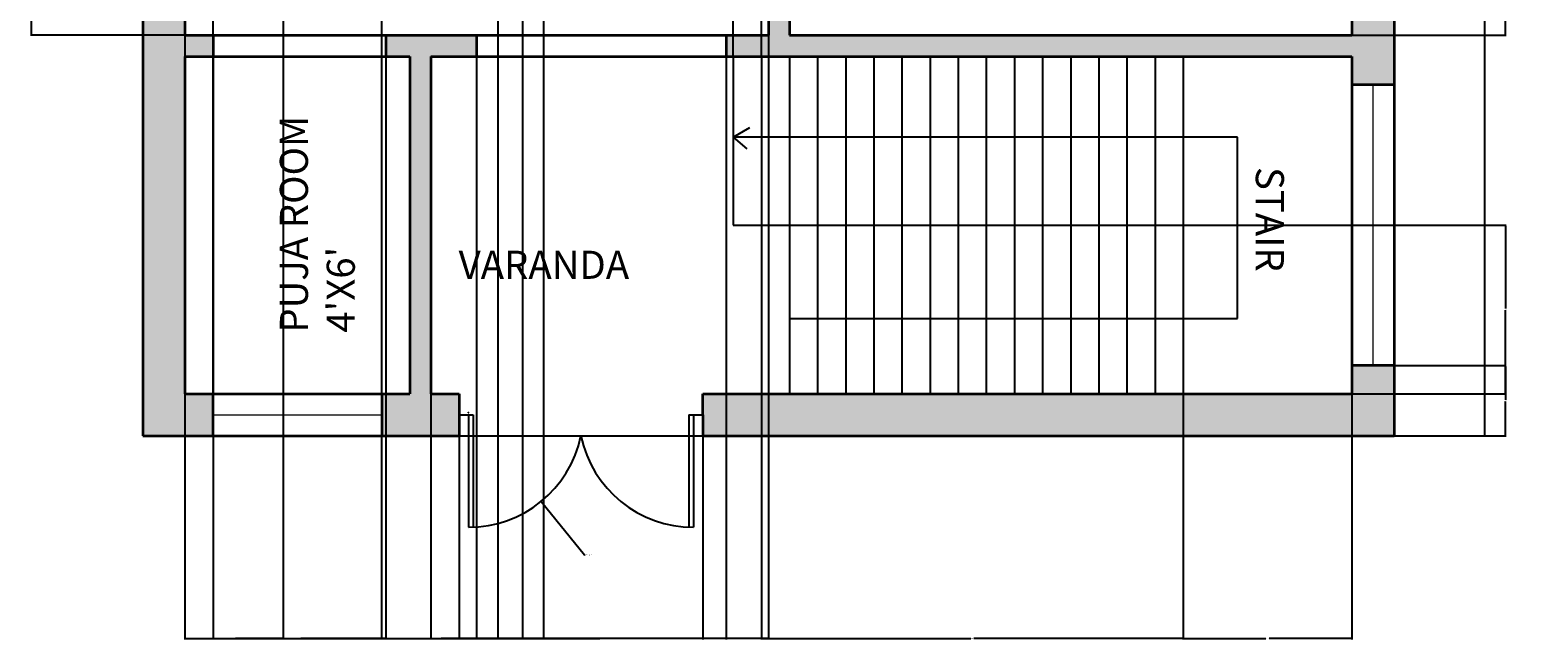
# Model space of a CAD drawing. Units: inches. Extents: x 10 to 332, y -471 to 73.
# Tile 1 of 5: x 10 to 332, y -471 to -341. Entities that reach past the tile are written whole.
import ezdxf

# ---------------------------------------------------------------- set-up
doc = ezdxf.new("R2010")
doc.units = ezdxf.units.IN
doc.header["$MEASUREMENT"] = 0
for name, color, linetype, lineweight in [('A-ANNO-DIMS', 2, 'Continuous', 18), ('A-AREA-IDEN', 7, 'Continuous', 18), ('A-DOOR', 3, 'Continuous', 25), ('A-FLOR-STRS', 7, 'Continuous', 25), ('A-GLAZ', 4, 'Continuous', 18), ('A-WALL', 7, 'Continuous', 35), ('A-WALL-PATT', 8, 'Continuous', 13)]:
    doc.layers.add(name, color=color, linetype=linetype, lineweight=lineweight)
doc.styles.get("Standard").update_dxf_attribs({"font": 'arial.ttf'})
doc.dimstyles.get("Standard").update_dxf_attribs({"dimtxt": 0.18, "dimasz": 0.18, "dimexe": 0.18, "dimexo": 0.0625, "dimgap": 0.09, "dimtad": 0, "dimtih": 1, "dimtoh": 1, "dimdec": 0, "dimzin": 0, "dimdsep": 46, "dimlunit": 3, "dimtxsty": 'Standard', "dimcen": 0.09, "dimadec": 0, "dimazin": 0, "dimtfac": 1, "dimtdec": 0, "dimtofl": 0, "dimtmove": 0, "dimatfit": 3, "dimfxl": 1, "dimtolj": 1, "dimtzin": 0, "dimarcsym": 0})

# ---------------------------------------------------------------- blocks, each defined once
blk = doc.blocks.new('*D3')
at = {"layer": 'A-ANNO-DIMS', "color": 0, "lineweight": -2, "transparency": 16777216}
for p, q in [((301.43, 11.99), (320.92, 11.99)), ((320.74, 11.81), (320.74, -204.61)), ((320.74, -427.33), (320.74, -210.92)), ((301.43, -427.51), (320.92, -427.51))]:
    blk.add_line(p, q, dxfattribs=at)
at = {"layer": 'A-ANNO-DIMS', "color": 0, "transparency": 16777216}
for points in [[(320.71, 11.81), (320.77, 11.81), (320.74, 11.99)], [(320.71, -427.33), (320.77, -427.33), (320.74, -427.51)]]:
    blk.add_solid(points, dxfattribs=at)
at = {"layer": 'Defpoints', "color": 0, "transparency": 16777216}
for p in [(301.37, 11.99), (301.37, -427.51), (320.74, -427.51)]:
    blk.add_point(p, dxfattribs=at)
at = {"layer": 'A-ANNO-DIMS', "color": 0, "transparency": 16777216, "insert": (320.74, -207.76), "char_height": 6, "attachment_point": 5}
blk.add_mtext('\\A1;36\'-8"', dxfattribs=at)
blk = doc.blocks.new('WIN-60')
for p, q in [((0, 9), (60, 9)), ((0, 4.5), (60, 4.5)), ((60, 0), (0, 0))]:
    blk.add_line(p, q)
blk = doc.blocks.new('*D30')
at = {"layer": 'A-ANNO-DIMS', "color": 0, "lineweight": -2, "transparency": 16777216}
for p, q in [((167.87, -93.08), (167.87, -470.94)), ((43.37, -97.58), (43.37, -470.94)), ((43.55, -470.76), (105.02, -470.76)), ((167.69, -470.76), (106.22, -470.76))]:
    blk.add_line(p, q, dxfattribs=at)
at = {"layer": 'A-ANNO-DIMS', "color": 0, "transparency": 16777216}
for points in [[(43.55, -470.73), (43.55, -470.79), (43.37, -470.76)], [(167.69, -470.73), (167.69, -470.79), (167.87, -470.76)]]:
    blk.add_solid(points, dxfattribs=at)
at = {"layer": 'Defpoints', "color": 0, "transparency": 16777216}
for p in [(167.87, -93.01), (43.37, -97.51), (167.87, -470.76)]:
    blk.add_point(p, dxfattribs=at)
at = {"layer": 'A-ANNO-DIMS', "color": 0, "transparency": 16777216, "insert": (105.62, -470.76), "char_height": 0.18, "attachment_point": 5}
blk.add_mtext('\\A1;10\'-4 1/2"', dxfattribs=at)
blk = doc.blocks.new('*D31')
at = {"layer": 'A-ANNO-DIMS', "color": 0, "lineweight": -2, "transparency": 16777216}
for p, q in [((43.3, -225.2), (10.44, -225.2)), ((10.62, -225.38), (10.62, -283.43)), ((10.62, -341.83), (10.62, -283.79)), ((43.3, -342.01), (10.44, -342.01))]:
    blk.add_line(p, q, dxfattribs=at)
at = {"layer": 'A-ANNO-DIMS', "color": 0, "transparency": 16777216}
for points in [[(10.59, -225.38), (10.65, -225.38), (10.62, -225.2)], [(10.59, -341.83), (10.65, -341.83), (10.62, -342.01)]]:
    blk.add_solid(points, dxfattribs=at)
at = {"layer": 'Defpoints', "color": 0, "transparency": 16777216}
for p in [(43.37, -225.2), (10.62, -342.01), (43.37, -342.01)]:
    blk.add_point(p, dxfattribs=at)
at = {"layer": 'A-ANNO-DIMS', "color": 0, "transparency": 16777216, "insert": (10.62, -283.61), "char_height": 0.18, "attachment_point": 5}
blk.add_mtext('\\A1;9\'-9"', dxfattribs=at)
blk = doc.blocks.new('*D32')
at = {"layer": 'A-ANNO-DIMS', "color": 0, "lineweight": -2, "transparency": 16777216}
for p, q in [((101.87, -427.58), (101.87, -470.94)), ((153.87, -427.58), (153.87, -470.94)), ((102.05, -470.76), (127.53, -470.76)), ((153.69, -470.76), (128.2, -470.76))]:
    blk.add_line(p, q, dxfattribs=at)
at = {"layer": 'A-ANNO-DIMS', "color": 0, "transparency": 16777216}
for points in [[(102.05, -470.73), (102.05, -470.79), (101.87, -470.76)], [(153.69, -470.73), (153.69, -470.79), (153.87, -470.76)]]:
    blk.add_solid(points, dxfattribs=at)
at = {"layer": 'Defpoints', "color": 0, "transparency": 16777216}
for p in [(101.87, -427.51), (153.87, -427.51), (153.87, -470.76)]:
    blk.add_point(p, dxfattribs=at)
at = {"layer": 'A-ANNO-DIMS', "color": 0, "transparency": 16777216, "insert": (127.87, -470.76), "char_height": 0.18, "attachment_point": 5}
blk.add_mtext('\\A1;4\'-4"', dxfattribs=at)
blk = doc.blocks.new('*D33')
at = {"layer": 'A-ANNO-DIMS', "color": 0, "lineweight": -2, "transparency": 16777216}
for p, q in [((95.87, -418.58), (95.87, -470.94)), ((101.87, -418.58), (101.87, -470.94)), ((96.05, -470.76), (98.54, -470.76)), ((101.69, -470.76), (99.2, -470.76))]:
    blk.add_line(p, q, dxfattribs=at)
at = {"layer": 'A-ANNO-DIMS', "color": 0, "transparency": 16777216}
for points in [[(96.05, -470.73), (96.05, -470.79), (95.87, -470.76)], [(101.69, -470.73), (101.69, -470.79), (101.87, -470.76)]]:
    blk.add_solid(points, dxfattribs=at)
at = {"layer": 'Defpoints', "color": 0, "transparency": 16777216}
for p in [(95.87, -418.51), (101.87, -418.51), (101.87, -470.76)]:
    blk.add_point(p, dxfattribs=at)
at = {"layer": 'A-ANNO-DIMS', "color": 0, "transparency": 16777216, "insert": (98.87, -470.76), "char_height": 0.18, "attachment_point": 5}
blk.add_mtext('\\A1;0\'-6"', dxfattribs=at)
blk = doc.blocks.new('*D34')
at = {"layer": 'A-ANNO-DIMS', "color": 0, "lineweight": -2, "transparency": 16777216}
for p, q in [((166.37, -418.58), (166.37, -470.94)), ((256.37, -418.58), (256.37, -470.94)), ((166.55, -470.76), (211.04, -470.76)), ((256.19, -470.76), (211.69, -470.76))]:
    blk.add_line(p, q, dxfattribs=at)
at = {"layer": 'A-ANNO-DIMS', "color": 0, "transparency": 16777216}
for points in [[(166.55, -470.73), (166.55, -470.79), (166.37, -470.76)], [(256.19, -470.73), (256.19, -470.79), (256.37, -470.76)]]:
    blk.add_solid(points, dxfattribs=at)
at = {"layer": 'Defpoints', "color": 0, "transparency": 16777216}
for p in [(166.37, -418.51), (256.37, -418.51), (256.37, -470.76)]:
    blk.add_point(p, dxfattribs=at)
at = {"layer": 'A-ANNO-DIMS', "color": 0, "transparency": 16777216, "insert": (211.37, -470.76), "char_height": 0.18, "attachment_point": 5}
blk.add_mtext('\\A1;7\'-6"', dxfattribs=at)
blk = doc.blocks.new('*D35')
at = {"layer": 'A-ANNO-DIMS', "color": 0, "lineweight": -2, "transparency": 16777216}
for p, q in [((256.37, -418.58), (256.37, -470.94)), ((292.37, -418.58), (292.37, -470.94)), ((256.55, -470.76), (274.04, -470.76)), ((292.19, -470.76), (274.7, -470.76))]:
    blk.add_line(p, q, dxfattribs=at)
at = {"layer": 'A-ANNO-DIMS', "color": 0, "transparency": 16777216}
for points in [[(256.55, -470.73), (256.55, -470.79), (256.37, -470.76)], [(292.19, -470.73), (292.19, -470.79), (292.37, -470.76)]]:
    blk.add_solid(points, dxfattribs=at)
at = {"layer": 'Defpoints', "color": 0, "transparency": 16777216}
for p in [(256.37, -418.51), (292.37, -418.51), (292.37, -470.76)]:
    blk.add_point(p, dxfattribs=at)
at = {"layer": 'A-ANNO-DIMS', "color": 0, "transparency": 16777216, "insert": (274.37, -470.76), "char_height": 0.18, "attachment_point": 5}
blk.add_mtext('\\A1;3\'-0"', dxfattribs=at)
blk = doc.blocks.new('*D36')
at = {"layer": 'A-ANNO-DIMS', "color": 0, "lineweight": -2, "transparency": 16777216}
for p, q in [((160.37, -346.45), (160.37, 35.92)), ((160.55, 35.74), (163.04, 35.74)), ((166.19, 35.74), (163.7, 35.74)), ((166.37, -346.45), (166.37, 35.92))]:
    blk.add_line(p, q, dxfattribs=at)
at = {"layer": 'A-ANNO-DIMS', "color": 0, "transparency": 16777216}
for points in [[(160.55, 35.77), (160.55, 35.71), (160.37, 35.74)], [(166.19, 35.77), (166.19, 35.71), (166.37, 35.74)]]:
    blk.add_solid(points, dxfattribs=at)
at = {"layer": 'Defpoints', "color": 0, "transparency": 16777216}
for p in [(166.37, 35.74), (160.37, -346.51), (166.37, -346.51)]:
    blk.add_point(p, dxfattribs=at)
at = {"layer": 'A-ANNO-DIMS', "color": 0, "transparency": 16777216, "insert": (163.37, 35.74), "char_height": 0.18, "attachment_point": 5}
blk.add_mtext('\\A1;0\'-6"', dxfattribs=at)
blk = doc.blocks.new('*D44')
at = {"layer": 'A-ANNO-DIMS', "color": 0, "lineweight": -2, "transparency": 16777216}
for p, q in [((292.43, -312.01), (325.3, -312.01)), ((325.12, -312.19), (325.12, -326.83)), ((325.12, -341.83), (325.12, -327.2)), ((292.43, -342.01), (325.3, -342.01))]:
    blk.add_line(p, q, dxfattribs=at)
at = {"layer": 'A-ANNO-DIMS', "color": 0, "transparency": 16777216}
for points in [[(325.09, -312.19), (325.15, -312.19), (325.12, -312.01)], [(325.09, -341.83), (325.15, -341.83), (325.12, -342.01)]]:
    blk.add_solid(points, dxfattribs=at)
at = {"layer": 'Defpoints', "color": 0, "transparency": 16777216}
for p in [(292.37, -312.01), (292.37, -342.01), (325.12, -342.01)]:
    blk.add_point(p, dxfattribs=at)
at = {"layer": 'A-ANNO-DIMS', "color": 0, "transparency": 16777216, "insert": (325.12, -327.01), "char_height": 0.18, "attachment_point": 5}
blk.add_mtext('\\A1;2\'-6"', dxfattribs=at)
blk = doc.blocks.new('*D45')
at = {"layer": 'A-ANNO-DIMS', "color": 0, "lineweight": -2, "transparency": 16777216}
for p, q in [((301.43, -412.51), (325.3, -412.51)), ((325.12, -412.69), (325.12, -419.83)), ((325.12, -427.33), (325.12, -420.2)), ((301.43, -427.51), (325.3, -427.51))]:
    blk.add_line(p, q, dxfattribs=at)
at = {"layer": 'A-ANNO-DIMS', "color": 0, "transparency": 16777216}
for points in [[(325.09, -412.69), (325.15, -412.69), (325.12, -412.51)], [(325.09, -427.33), (325.15, -427.33), (325.12, -427.51)]]:
    blk.add_solid(points, dxfattribs=at)
at = {"layer": 'Defpoints', "color": 0, "transparency": 16777216}
for p in [(301.37, -412.51), (301.37, -427.51), (325.12, -427.51)]:
    blk.add_point(p, dxfattribs=at)
at = {"layer": 'A-ANNO-DIMS', "color": 0, "transparency": 16777216, "insert": (325.12, -420.01), "char_height": 0.18, "attachment_point": 5}
blk.add_mtext('\\A1;1\'-3"', dxfattribs=at)
blk = doc.blocks.new('*D46')
at = {"layer": 'A-ANNO-DIMS', "color": 0, "lineweight": -2, "transparency": 16777216}
for p, q in [((43.37, -93.08), (43.37, -470.94)), ((64.36, -93.08), (64.36, -470.94)), ((43.55, -470.76), (53.54, -470.76)), ((64.18, -470.76), (54.18, -470.76))]:
    blk.add_line(p, q, dxfattribs=at)
at = {"layer": 'A-ANNO-DIMS', "color": 0, "transparency": 16777216}
for points in [[(43.55, -470.73), (43.55, -470.79), (43.37, -470.76)], [(64.18, -470.73), (64.18, -470.79), (64.36, -470.76)]]:
    blk.add_solid(points, dxfattribs=at)
at = {"layer": 'Defpoints', "color": 0, "transparency": 16777216}
for p in [(43.37, -93.01), (64.36, -93.01), (64.36, -470.76)]:
    blk.add_point(p, dxfattribs=at)
at = {"layer": 'A-ANNO-DIMS', "color": 0, "transparency": 16777216, "insert": (53.86, -470.76), "char_height": 0.18, "attachment_point": 5}
blk.add_mtext('\\A1;1\'-9"', dxfattribs=at)
blk = doc.blocks.new('*D48')
at = {"layer": 'A-ANNO-DIMS', "color": 0, "lineweight": -2, "transparency": 16777216}
for p, q in [((85.3, -93.08), (85.3, -470.94)), ((110.16, -93.08), (110.16, -470.94)), ((85.48, -470.76), (97.4, -470.76)), ((109.98, -470.76), (98.06, -470.76))]:
    blk.add_line(p, q, dxfattribs=at)
at = {"layer": 'A-ANNO-DIMS', "color": 0, "transparency": 16777216}
for points in [[(85.48, -470.73), (85.48, -470.79), (85.3, -470.76)], [(109.98, -470.73), (109.98, -470.79), (110.16, -470.76)]]:
    blk.add_solid(points, dxfattribs=at)
at = {"layer": 'Defpoints', "color": 0, "transparency": 16777216}
for p in [(85.3, -93.01), (110.16, -93.01), (110.16, -470.76)]:
    blk.add_point(p, dxfattribs=at)
at = {"layer": 'A-ANNO-DIMS', "color": 0, "transparency": 16777216, "insert": (97.73, -470.76), "char_height": 0.18, "attachment_point": 5}
blk.add_mtext('\\A1;2\'-1"', dxfattribs=at)
blk = doc.blocks.new('*D50')
at = {"layer": 'A-ANNO-DIMS', "color": 0, "lineweight": -2, "transparency": 16777216}
for p, q in [((115.37, -93.08), (115.37, -470.94)), ((119.87, -97.58), (119.87, -470.94)), ((115.55, -470.76), (117.08, -470.76)), ((119.69, -470.76), (118.16, -470.76))]:
    blk.add_line(p, q, dxfattribs=at)
at = {"layer": 'A-ANNO-DIMS', "color": 0, "transparency": 16777216}
for points in [[(115.55, -470.73), (115.55, -470.79), (115.37, -470.76)], [(119.69, -470.73), (119.69, -470.79), (119.87, -470.76)]]:
    blk.add_solid(points, dxfattribs=at)
at = {"layer": 'Defpoints', "color": 0, "transparency": 16777216}
for p in [(115.37, -93.01), (119.87, -97.51), (119.87, -470.76)]:
    blk.add_point(p, dxfattribs=at)
at = {"layer": 'A-ANNO-DIMS', "color": 0, "transparency": 16777216, "insert": (117.62, -470.76), "char_height": 0.18, "attachment_point": 5}
blk.add_mtext('\\A1;0\'-4 1/2"', dxfattribs=at)
blk = doc.blocks.new('*D54')
at = {"layer": 'A-ANNO-DIMS', "color": 0, "lineweight": -2, "transparency": 16777216}
for p, q in [((49.37, -418.45), (49.37, 35.92)), ((49.55, 35.74), (67.04, 35.74)), ((85.19, 35.74), (67.7, 35.74)), ((85.37, -418.45), (85.37, 35.92))]:
    blk.add_line(p, q, dxfattribs=at)
at = {"layer": 'A-ANNO-DIMS', "color": 0, "transparency": 16777216}
for points in [[(49.55, 35.77), (49.55, 35.71), (49.37, 35.74)], [(85.19, 35.77), (85.19, 35.71), (85.37, 35.74)]]:
    blk.add_solid(points, dxfattribs=at)
at = {"layer": 'Defpoints', "color": 0, "transparency": 16777216}
for p in [(85.37, 35.74), (49.37, -418.51), (85.37, -418.51)]:
    blk.add_point(p, dxfattribs=at)
at = {"layer": 'A-ANNO-DIMS', "color": 0, "transparency": 16777216, "insert": (67.37, 35.74), "char_height": 0.18, "attachment_point": 5}
blk.add_mtext('\\A1;3\'-0"', dxfattribs=at)
blk = doc.blocks.new('*D60')
at = {"layer": 'A-ANNO-DIMS', "color": 0, "lineweight": -2, "transparency": 16777216}
for p, q in [((49.4, -342.08), (49.4, -470.94)), ((86.21, -342.08), (86.21, -470.94)), ((49.58, -470.76), (67.48, -470.76)), ((86.03, -470.76), (68.13, -470.76))]:
    blk.add_line(p, q, dxfattribs=at)
at = {"layer": 'A-ANNO-DIMS', "color": 0, "transparency": 16777216}
for points in [[(49.58, -470.73), (49.58, -470.79), (49.4, -470.76)], [(86.03, -470.73), (86.03, -470.79), (86.21, -470.76)]]:
    blk.add_solid(points, dxfattribs=at)
at = {"layer": 'Defpoints', "color": 0, "transparency": 16777216}
for p in [(49.4, -342.01), (86.21, -342.01), (86.21, -470.76)]:
    blk.add_point(p, dxfattribs=at)
at = {"layer": 'A-ANNO-DIMS', "color": 0, "transparency": 16777216, "insert": (67.81, -470.76), "char_height": 0.18, "attachment_point": 5}
blk.add_mtext('\\A1;3\'-1"', dxfattribs=at)
blk = doc.blocks.new('*D61')
at = {"layer": 'A-ANNO-DIMS', "color": 0, "lineweight": -2, "transparency": 16777216}
for p, q in [((105.62, -342.08), (105.62, -470.94)), ((158.84, -342.08), (158.84, -470.94)), ((105.8, -470.76), (131.9, -470.76)), ((158.66, -470.76), (132.56, -470.76))]:
    blk.add_line(p, q, dxfattribs=at)
at = {"layer": 'A-ANNO-DIMS', "color": 0, "transparency": 16777216}
for points in [[(105.8, -470.73), (105.8, -470.79), (105.62, -470.76)], [(158.66, -470.73), (158.66, -470.79), (158.84, -470.76)]]:
    blk.add_solid(points, dxfattribs=at)
at = {"layer": 'Defpoints', "color": 0, "transparency": 16777216}
for p in [(105.62, -342.01), (158.84, -342.01), (158.84, -470.76)]:
    blk.add_point(p, dxfattribs=at)
at = {"layer": 'A-ANNO-DIMS', "color": 0, "transparency": 16777216, "insert": (132.23, -470.76), "char_height": 0.18, "attachment_point": 5}
blk.add_mtext('\\A1;4\'-5"', dxfattribs=at)
blk = doc.blocks.new('*D62')
at = {"layer": 'A-ANNO-DIMS', "color": 0, "lineweight": -2, "transparency": 16777216}
for p, q in [((256.43, -382.51), (325.3, -382.51)), ((325.12, -382.69), (325.12, -400.33)), ((325.12, -418.33), (325.12, -400.7)), ((256.43, -418.51), (325.3, -418.51))]:
    blk.add_line(p, q, dxfattribs=at)
at = {"layer": 'A-ANNO-DIMS', "color": 0, "transparency": 16777216}
for points in [[(325.09, -382.69), (325.15, -382.69), (325.12, -382.51)], [(325.09, -418.33), (325.15, -418.33), (325.12, -418.51)]]:
    blk.add_solid(points, dxfattribs=at)
at = {"layer": 'Defpoints', "color": 0, "transparency": 16777216}
for p in [(256.37, -382.51), (256.37, -418.51), (325.12, -418.51)]:
    blk.add_point(p, dxfattribs=at)
at = {"layer": 'A-ANNO-DIMS', "color": 0, "transparency": 16777216, "insert": (325.12, -400.51), "char_height": 0.18, "attachment_point": 5}
blk.add_mtext('\\A1;3\'-0"', dxfattribs=at)
blk = doc.blocks.new('*D63')
at = {"layer": 'A-ANNO-DIMS', "color": 0, "lineweight": -2, "transparency": 16777216}
for p, q in [((103.78, -422.5), (103.96, -422.5)), ((103.87, -422.59), (103.87, -422.41)), ((128.61, -452.94), (119.44, -441.67)), ((128.79, -452.94), (128.61, -452.94))]:
    blk.add_line(p, q, dxfattribs=at)
at = {"layer": 'A-ANNO-DIMS', "color": 0, "transparency": 16777216}
blk.add_solid([(119.47, -441.65), (119.42, -441.68), (119.33, -441.53)], dxfattribs=at)
at = {"layer": 'Defpoints', "color": 0, "transparency": 16777216}
for p in [(103.87, -422.5), (119.33, -441.53)]:
    blk.add_point(p, dxfattribs=at)
at = {"layer": 'A-ANNO-DIMS', "color": 0, "transparency": 16777216, "insert": (129.61, -452.94), "char_height": 0.18, "attachment_point": 5}
blk.add_mtext('\\A1;2X R2\'-0 1/2"', dxfattribs=at)

msp = doc.modelspace()

# ---------------------------------------------------------------- hatches: boundary and pattern name
at = {"layer": 'A-WALL-PATT'}
h = msp.add_hatch(color=256, dxfattribs=at)
h.dxf.hatch_style = 1
h.paths.add_polyline_path([(132.66, 11.99), (109.37, 11.99), (109.37, 2.99), (115.37, 2.99), (115.37, -93.01), (110.16, -93.01), (110.16, -97.51), (119.87, -97.51), (119.87, -73.51), (167.87, -73.51), (167.87, -107.01), (170.12, -107.01), (172.37, -107.01), (172.37, -63.01), (167.87, -63.01), (167.87, -69.01), (119.87, -69.01), (119.87, 2.99), (132.66, 2.99)])
h.paths.add_polyline_path([(202.37, 11.99), (152.96, 11.99), (152.96, 2.99), (167.87, 2.99), (167.87, -35.01), (170.12, -35.01), (172.37, -35.01), (172.37, 2.99), (202.37, 2.99)])
h.paths.add_polyline_path([(49.37, 11.99), (34.37, 11.99), (34.37, -15.01), (43.37, -15.01), (43.37, 2.99), (49.37, 2.99)])
h.paths.add_polyline_path([(301.37, 11.99), (262.37, 11.99), (262.37, 2.99), (292.37, 2.99), (292.37, -39.01), (301.37, -39.01)])
h.paths.add_polyline_path([(85.3, -93.01), (43.37, -93.01), (43.37, -75.01), (34.37, -75.01), (34.37, -165.2), (43.37, -165.2), (43.37, -97.51), (85.3, -97.51)])
h.paths.add_polyline_path([(43.37, -225.2), (34.37, -225.2), (34.37, -427.51), (49.37, -427.51), (49.37, -418.51), (43.37, -418.51), (43.37, -346.51), (49.4, -346.51), (49.4, -342.01), (43.37, -342.01)])
h.paths.add_polyline_path([(105.62, -342.01), (86.21, -342.01), (86.21, -346.51), (91.37, -346.51), (91.37, -418.51), (85.37, -418.51), (85.37, -427.51), (101.87, -427.51), (101.87, -418.51), (95.87, -418.51), (95.87, -346.51), (105.62, -346.51)])
h.paths.add_polyline_path([(301.37, -312.01), (292.37, -312.01), (292.37, -342.01), (172.37, -342.01), (172.37, -179.51), (170.12, -179.51), (167.87, -179.51), (167.87, -342.01), (158.84, -342.01), (158.84, -346.51), (292.37, -346.51), (292.37, -352.51), (301.37, -352.51)])
h.paths.add_polyline_path([(301.37, -412.51), (292.37, -412.51), (292.37, -418.51), (153.87, -418.51), (153.87, -423.01), (153.87, -427.51), (301.37, -427.51)])
h.paths.add_polyline_path([(301.37, -99.01), (292.37, -99.01), (292.37, -141.01), (172.37, -141.01), (172.37, -135.01), (167.87, -135.01), (167.87, -151.51), (172.37, -151.51), (172.37, -145.51), (292.37, -145.51), (292.37, -165.79), (301.37, -165.79)])

# ---------------------------------------------------------------- linework, layer by layer
at = {"layer": 'A-DOOR'}
for p, q in [((101.87, -423.01), (103.87, -423.01)), ((103.87, -423.01), (103.87, -447.01)), ((103.87, -423.01), (104.87, -423.01)), ((104.87, -423.01), (104.87, -447.01)), ((150.87, -423.01), (150.87, -447.01)), ((150.87, -423.01), (151.87, -423.01)), ((151.87, -423.01), (153.87, -423.01)), ((151.87, -423.01), (151.87, -447.01)), ((101.87, -427.51), (153.87, -427.51))]:
    msp.add_line(p, q, dxfattribs=at)
for centre, start, end in [((103.87, -422.5), 270, 348.1877), ((151.87, -422.5), 191.8123, 270)]:
    msp.add_arc(centre, 24.52, start, end, dxfattribs=at)
at = {"layer": 'A-FLOR-STRS'}
for p, q in [((160.37, -346.51), (160.37, -382.51)), ((166.37, -346.51), (166.37, -418.51)), ((172.37, -346.51), (172.37, -418.51)), ((178.37, -346.51), (178.37, -418.51)), ((184.37, -346.51), (184.37, -418.51)), ((190.37, -346.51), (190.37, -418.51)), ((196.37, -346.51), (196.37, -418.51)), ((202.37, -346.51), (202.37, -418.51)), ((208.37, -346.51), (208.37, -418.51)), ((214.37, -346.51), (214.37, -418.51)), ((220.37, -346.51), (220.37, -418.51)), ((226.37, -346.51), (226.37, -418.51)), ((232.37, -346.51), (232.37, -418.51)), ((238.37, -346.51), (238.37, -418.51)), ((244.37, -346.51), (244.37, -418.51)), ((250.37, -346.51), (250.37, -418.51)), ((256.37, -346.51), (256.37, -418.51)), ((160.37, -363.73), (163.91, -361.71)), ((267.99, -363.73), (160.37, -363.73)), ((160.37, -363.73), (163.3, -366.22)), ((267.99, -402.43), (267.99, -363.73)), ((160.37, -382.51), (256.37, -382.51)), ((172.37, -402.43), (267.99, -402.43))]:
    msp.add_line(p, q, dxfattribs=at)
at = {"layer": 'A-GLAZ'}
for p, q in [((49.37, -418.51), (85.37, -418.51)), ((49.37, -423.01), (85.37, -423.01)), ((85.37, -427.51), (49.37, -427.51))]:
    msp.add_line(p, q, dxfattribs=at)
at = {"layer": 'A-WALL'}
for p, q in [((34.37, 11.99), (34.37, -427.51)), ((301.37, 11.99), (301.37, -427.51)), ((43.37, -97.51), (43.37, -342.01)), ((167.87, -179.51), (167.87, -342.01)), ((172.37, -179.51), (172.37, -342.01)), ((292.37, -222.01), (292.37, -342.01)), ((43.37, -342.01), (167.87, -342.01)), ((49.4, -342.01), (49.4, -346.51)), ((86.21, -342.01), (86.21, -346.51)), ((105.62, -342.01), (105.62, -346.51)), ((158.84, -342.01), (158.84, -346.51)), ((172.37, -342.01), (292.37, -342.01)), ((43.37, -346.51), (91.37, -346.51)), ((43.37, -346.51), (43.37, -418.51)), ((91.37, -346.51), (91.37, -418.51)), ((95.87, -346.51), (95.87, -418.51)), ((95.87, -346.51), (292.37, -346.51)), ((292.37, -346.51), (292.37, -418.51)), ((292.37, -352.51), (301.37, -352.51)), ((301.37, -412.51), (292.37, -412.51)), ((43.37, -418.51), (91.37, -418.51)), ((49.37, -427.51), (49.37, -418.51)), ((85.37, -418.51), (85.37, -427.51)), ((95.87, -418.51), (101.87, -418.51)), ((101.87, -418.51), (101.87, -427.51)), ((153.87, -423.01), (153.87, -418.51)), ((153.87, -418.51), (292.37, -418.51)), ((153.87, -423.01), (153.87, -427.51)), ((34.37, -427.51), (101.87, -427.51)), ((153.87, -427.51), (301.37, -427.51))]:
    msp.add_line(p, q, dxfattribs=at)

# ---------------------------------------------------------------- block references
at = {"layer": 'A-GLAZ', "rotation": 270}
msp.add_blockref('WIN-60', (292.37, -352.51), dxfattribs=at)

# ---------------------------------------------------------------- texts
at = {"layer": 'A-AREA-IDEN', "char_height": 6, "attachment_point": 1}
for s, insert, rotation in [("PUJA ROOM\\P4'X6'", (63.62, -405.47), 90), ('STAIR', (277.87, -370.12), 270)]:
    msp.add_mtext(s, dxfattribs=dict(at, insert=insert, rotation=rotation))
at = {"layer": 'A-AREA-IDEN', "insert": (101.77, -387.99), "char_height": 6, "attachment_point": 1}
msp.add_mtext('VARANDA', dxfattribs=at)

# ---------------------------------------------------------------- dimensions: what is measured, and where the dimension line sits
at = {"layer": 'A-ANNO-DIMS'}
for base, p1, p2, picture, middle in [((85.37, 35.74), (49.37, -418.51), (85.37, -418.51), '*D54', (67.37, 35.74)), ((166.37, 35.74), (160.37, -346.51), (166.37, -346.51), '*D36', (163.37, 35.74)), ((167.87, -470.76), (43.37, -97.51), (167.87, -93.01), '*D30', (105.62, -470.76)), ((64.36, -470.76), (43.37, -93.01), (64.36, -93.01), '*D46', (53.86, -470.76)), ((110.16, -470.76), (85.3, -93.01), (110.16, -93.01), '*D48', (97.73, -470.76)), ((119.87, -470.76), (115.37, -93.01), (119.87, -97.51), '*D50', (117.62, -470.76)), ((86.21, -470.76), (49.4, -342.01), (86.21, -342.01), '*D60', (67.81, -470.76)), ((158.84, -470.76), (105.62, -342.01), (158.84, -342.01), '*D61', (132.23, -470.76)), ((101.87, -470.76), (95.87, -418.51), (101.87, -418.51), '*D33', (98.87, -470.76)), ((256.37, -470.76), (166.37, -418.51), (256.37, -418.51), '*D34', (211.37, -470.76)), ((292.37, -470.76), (256.37, -418.51), (292.37, -418.51), '*D35', (274.37, -470.76)), ((153.87, -470.76), (101.87, -427.51), (153.87, -427.51), '*D32', (127.87, -470.76))]:
    dim = msp.add_linear_dim(base=base, p1=p1, p2=p2, dimstyle='Standard', override={"dimdec": 1, "dimlfac": 1, "dimrnd": 0, "dimzin": 1, "dimdsep": 46, "dimlunit": 4, "dimfrac": 2}, dxfattribs=at)
    dim.commit()
    dim.dimension.update_dxf_attribs({"geometry": picture, "text_midpoint": middle})
for base, p1, p2, override, picture, middle in [((320.73862044, -427.51494379), (301.36648826, 11.98505621), (301.36648826, -427.51494379), {"dimtxt": 6, "dimclrd": 0, "dimclre": 0, "dimclrt": 0}, '*D3', (320.73862044, -207.76494379)), ((10.62, -342.01), (43.37, -225.2), (43.37, -342.01), {"dimdec": 1, "dimlfac": 1, "dimrnd": 0, "dimzin": 1, "dimdsep": 46, "dimlunit": 4, "dimfrac": 2}, '*D31', (10.62, -283.61)), ((325.12, -342.01), (292.37, -312.01), (292.37, -342.01), {"dimdec": 1, "dimlfac": 1, "dimrnd": 0, "dimzin": 1, "dimdsep": 46, "dimlunit": 4, "dimfrac": 2}, '*D44', (325.12, -327.01)), ((325.12, -418.51), (256.37, -382.51), (256.37, -418.51), {"dimdec": 1, "dimlfac": 1, "dimrnd": 0, "dimzin": 1, "dimdsep": 46, "dimlunit": 4, "dimfrac": 2}, '*D62', (325.12, -400.51)), ((325.12, -427.51), (301.37, -412.51), (301.37, -427.51), {"dimdec": 1, "dimlfac": 1, "dimrnd": 0, "dimzin": 1, "dimdsep": 46, "dimlunit": 4, "dimfrac": 2}, '*D45', (325.12, -420.01))]:
    dim = msp.add_linear_dim(base=base, p1=p1, p2=p2, angle=90, dimstyle='Standard', override=override, dxfattribs=at)
    dim.commit()
    dim.dimension.update_dxf_attribs({"geometry": picture, "text_midpoint": middle})
dim = msp.add_radius_dim(center=(103.87, -422.5), mpoint=(119.33, -441.53), text='2X <>', dimstyle='Standard', override={"dimdec": 1, "dimlfac": 1, "dimrnd": 0, "dimzin": 1, "dimdsep": 46, "dimlunit": 4, "dimfrac": 2}, dxfattribs=at)
dim.commit()
dim.dimension.update_dxf_attribs({"geometry": '*D63', "text_midpoint": (129.61, -452.94), "dimtype": 164})

doc.saveas('drawing.dxf')
